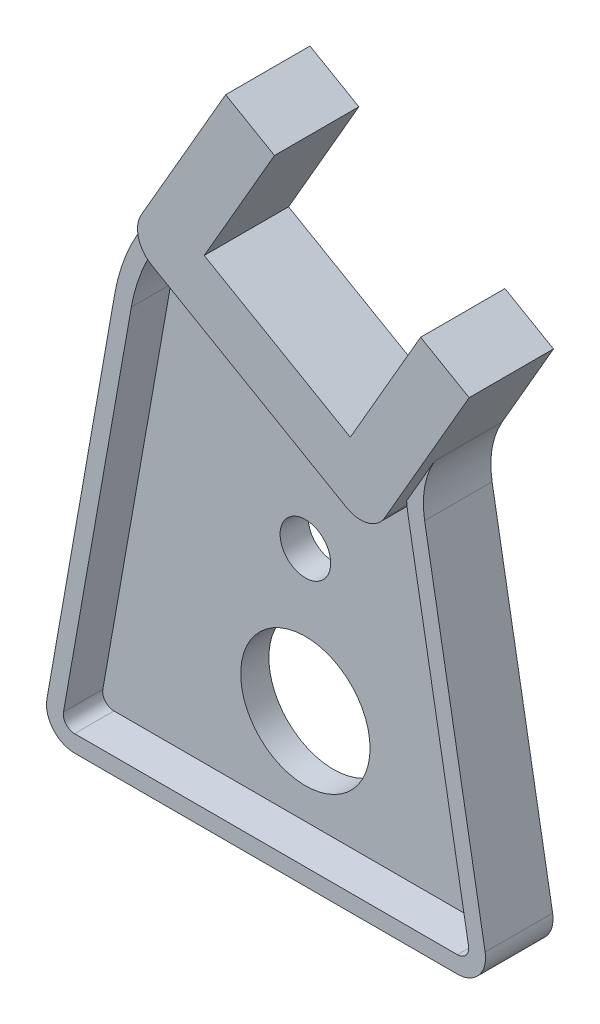
ISO-10303-21;
HEADER;
FILE_DESCRIPTION(('STEP AP214'),'2;1');
FILE_NAME('part.step','',(''),(''),'','','');
FILE_SCHEMA(('AUTOMOTIVE_DESIGN { 1 0 10303 214 1 1 1 1 }'));
ENDSEC;
DATA;
#1=APPLICATION_CONTEXT('core data for automotive mechanical design processes');
#2=APPLICATION_PROTOCOL_DEFINITION('international standard','automotive_design',2000,#1);
#3=PRODUCT_CONTEXT('',#1,'mechanical');
#4=PRODUCT('Part','Part','',(#3));
#5=PRODUCT_RELATED_PRODUCT_CATEGORY('part','',(#4));
#6=PRODUCT_DEFINITION_FORMATION('','',#4);
#7=PRODUCT_DEFINITION_CONTEXT('part definition',#1,'design');
#8=PRODUCT_DEFINITION('design','',#6,#7);
#9=PRODUCT_DEFINITION_SHAPE('','',#8);
#10=(LENGTH_UNIT() NAMED_UNIT(*) SI_UNIT(.MILLI.,.METRE.));
#11=(NAMED_UNIT(*) PLANE_ANGLE_UNIT() SI_UNIT($,.RADIAN.));
#12=(NAMED_UNIT(*) SI_UNIT($,.STERADIAN.) SOLID_ANGLE_UNIT());
#13=UNCERTAINTY_MEASURE_WITH_UNIT(LENGTH_MEASURE(1.E-05),#10,'distance_accuracy_value','');
#14=(GEOMETRIC_REPRESENTATION_CONTEXT(3) GLOBAL_UNCERTAINTY_ASSIGNED_CONTEXT((#13)) GLOBAL_UNIT_ASSIGNED_CONTEXT((#10,
#11,#12)) REPRESENTATION_CONTEXT('',''));
#15=CARTESIAN_POINT('',(0.,0.,0.));
#16=DIRECTION('',(0.,0.,1.));
#17=DIRECTION('',(1.,0.,0.));
#18=AXIS2_PLACEMENT_3D('',#15,#16,#17);
#19=CARTESIAN_POINT('',(0.,45.,12.));
#20=DIRECTION('',(0.,0.,-1.));
#21=DIRECTION('',(-1.,0.,0.));
#22=AXIS2_PLACEMENT_3D('',#19,#20,#21);
#23=CYLINDRICAL_SURFACE('',#22,4.5);
#24=CARTESIAN_POINT('',(0.,45.,0.));
#25=DIRECTION('',(0.,0.,1.));
#26=DIRECTION('',(1.,0.,0.));
#27=AXIS2_PLACEMENT_3D('',#24,#25,#26);
#28=CIRCLE('',#27,4.5);
#29=CARTESIAN_POINT('',(4.5,45.,0.));
#30=VERTEX_POINT('',#29);
#31=EDGE_CURVE('E350',#30,#30,#28,.T.);
#32=ORIENTED_EDGE('',*,*,#31,.F.);
#33=EDGE_LOOP('',(#32));
#34=FACE_BOUND('',#33,.T.);
#35=CARTESIAN_POINT('',(0.,45.,5.));
#36=DIRECTION('',(0.,0.,1.));
#37=DIRECTION('',(1.,0.,0.));
#38=AXIS2_PLACEMENT_3D('',#35,#36,#37);
#39=CIRCLE('',#38,4.5);
#40=CARTESIAN_POINT('',(4.5,45.,5.));
#41=VERTEX_POINT('',#40);
#42=EDGE_CURVE('E312',#41,#41,#39,.T.);
#43=ORIENTED_EDGE('',*,*,#42,.T.);
#44=EDGE_LOOP('',(#43));
#45=FACE_BOUND('',#44,.T.);
#46=ADVANCED_FACE('F41',(#34,#45),#23,.F.);
#47=CARTESIAN_POINT('',(0.,20.,12.));
#48=DIRECTION('',(0.,0.,-1.));
#49=DIRECTION('',(-1.,0.,0.));
#50=AXIS2_PLACEMENT_3D('',#47,#48,#49);
#51=CYLINDRICAL_SURFACE('',#50,11.5);
#52=CARTESIAN_POINT('',(0.,20.,0.));
#53=DIRECTION('',(0.,0.,1.));
#54=DIRECTION('',(1.,0.,0.));
#55=AXIS2_PLACEMENT_3D('',#52,#53,#54);
#56=CIRCLE('',#55,11.5);
#57=CARTESIAN_POINT('',(11.5,20.,0.));
#58=VERTEX_POINT('',#57);
#59=EDGE_CURVE('E318',#58,#58,#56,.T.);
#60=ORIENTED_EDGE('',*,*,#59,.F.);
#61=EDGE_LOOP('',(#60));
#62=FACE_BOUND('',#61,.T.);
#63=CARTESIAN_POINT('',(0.,20.,5.));
#64=DIRECTION('',(0.,0.,1.));
#65=DIRECTION('',(1.,0.,0.));
#66=AXIS2_PLACEMENT_3D('',#63,#64,#65);
#67=CIRCLE('',#66,11.5);
#68=CARTESIAN_POINT('',(11.5,20.,5.));
#69=VERTEX_POINT('',#68);
#70=EDGE_CURVE('E44',#69,#69,#67,.T.);
#71=ORIENTED_EDGE('',*,*,#70,.T.);
#72=EDGE_LOOP('',(#71));
#73=FACE_BOUND('',#72,.T.);
#74=ADVANCED_FACE('F555',(#62,#73),#51,.F.);
#75=CARTESIAN_POINT('',(-54.1549312273806,31.2663641220735,15.));
#76=DIRECTION('',(-0.866025403784441,0.499999999999996,0.));
#77=DIRECTION('',(-0.499999999999997,-0.866025403784441,0.));
#78=AXIS2_PLACEMENT_3D('',#75,#76,#77);
#79=PLANE('',#78);
#80=DIRECTION('',(0.499999999999996,0.866025403784441,0.));
#81=VECTOR('',#80,1.);
#82=CARTESIAN_POINT('',(-54.1549312273806,31.2663641220735,0.));
#83=LINE('',#82,#81);
#84=CARTESIAN_POINT('',(-22.7411868660834,85.6765654118211,0.));
#85=VERTEX_POINT('',#84);
#86=CARTESIAN_POINT('',(-4.17897858546452,117.827253254529,0.));
#87=VERTEX_POINT('',#86);
#88=EDGE_CURVE('E390',#85,#87,#83,.T.);
#89=ORIENTED_EDGE('',*,*,#88,.F.);
#90=DIRECTION('',(0.,0.,-1.));
#91=VECTOR('',#90,1.);
#92=CARTESIAN_POINT('',(-22.7411868660834,85.6765654118211,12.));
#93=LINE('',#92,#91);
#94=CARTESIAN_POINT('',(-22.7411868660834,85.6765654118211,12.));
#95=VERTEX_POINT('',#94);
#96=EDGE_CURVE('E374',#95,#85,#93,.T.);
#97=ORIENTED_EDGE('',*,*,#96,.F.);
#98=DIRECTION('',(0.499999999999996,0.866025403784441,0.));
#99=VECTOR('',#98,1.);
#100=CARTESIAN_POINT('',(-54.1549312273806,31.2663641220735,12.));
#101=LINE('',#100,#99);
#102=CARTESIAN_POINT('',(-19.1789785854643,91.846491140996,12.));
#103=VERTEX_POINT('',#102);
#104=EDGE_CURVE('E331',#95,#103,#101,.T.);
#105=ORIENTED_EDGE('',*,*,#104,.T.);
#106=DIRECTION('',(0.,0.,-1.));
#107=VECTOR('',#106,1.);
#108=CARTESIAN_POINT('',(-19.1789785854643,91.846491140996,15.));
#109=LINE('',#108,#107);
#110=CARTESIAN_POINT('',(-19.1789785854643,91.846491140996,15.));
#111=VERTEX_POINT('',#110);
#112=EDGE_CURVE('E11',#111,#103,#109,.T.);
#113=ORIENTED_EDGE('',*,*,#112,.F.);
#114=DIRECTION('',(0.499999999999996,0.866025403784441,0.));
#115=VECTOR('',#114,1.);
#116=CARTESIAN_POINT('',(-54.1549312273806,31.2663641220735,15.));
#117=LINE('',#116,#115);
#118=CARTESIAN_POINT('',(-4.17897858546452,117.827253254529,15.));
#119=VERTEX_POINT('',#118);
#120=EDGE_CURVE('E389',#111,#119,#117,.T.);
#121=ORIENTED_EDGE('',*,*,#120,.T.);
#122=DIRECTION('',(0.,0.,-1.));
#123=VECTOR('',#122,1.);
#124=CARTESIAN_POINT('',(-4.17897858546452,117.827253254529,15.));
#125=LINE('',#124,#123);
#126=EDGE_CURVE('E414',#119,#87,#125,.T.);
#127=ORIENTED_EDGE('',*,*,#126,.T.);
#128=EDGE_LOOP('',(#89,#97,#105,#113,#121,#127));
#129=FACE_BOUND('',#128,.T.);
#130=ADVANCED_FACE('F43',(#129),#79,.T.);
#131=CARTESIAN_POINT('',(-14.8488515665423,89.3464911409962,15.));
#132=DIRECTION('',(0.,0.,-1.));
#133=DIRECTION('',(-1.,0.,0.));
#134=AXIS2_PLACEMENT_3D('',#131,#132,#133);
#135=CYLINDRICAL_SURFACE('',#134,4.9999999999999);
#136=ORIENTED_EDGE('',*,*,#112,.T.);
#137=CARTESIAN_POINT('',(-14.8488515665423,89.3464911409962,12.));
#138=DIRECTION('',(0.,0.,1.));
#139=DIRECTION('',(1.,0.,0.));
#140=AXIS2_PLACEMENT_3D('',#137,#138,#139);
#141=CIRCLE('',#140,4.9999999999999);
#142=CARTESIAN_POINT('',(-18.8721898947694,86.3778637314644,12.));
#143=VERTEX_POINT('',#142);
#144=EDGE_CURVE('E335',#103,#143,#141,.T.);
#145=ORIENTED_EDGE('',*,*,#144,.T.);
#146=DIRECTION('',(0.,0.,1.));
#147=VECTOR('',#146,1.);
#148=CARTESIAN_POINT('',(-18.8721898947694,86.3778637314644,5.));
#149=LINE('',#148,#147);
#150=CARTESIAN_POINT('',(-18.8721898947694,86.3778637314644,5.));
#151=VERTEX_POINT('',#150);
#152=EDGE_CURVE('E280',#151,#143,#149,.T.);
#153=ORIENTED_EDGE('',*,*,#152,.F.);
#154=CARTESIAN_POINT('',(-14.8488515665423,89.3464911409962,5.));
#155=DIRECTION('',(0.,0.,-1.));
#156=DIRECTION('',(1.,0.,0.));
#157=AXIS2_PLACEMENT_3D('',#154,#155,#156);
#158=CIRCLE('',#157,5.00000000000019);
#159=CARTESIAN_POINT('',(-17.3488515665418,85.0163641220735,5.));
#160=VERTEX_POINT('',#159);
#161=EDGE_CURVE('E238',#160,#151,#158,.T.);
#162=ORIENTED_EDGE('',*,*,#161,.F.);
#163=DIRECTION('',(0.,0.,-1.));
#164=VECTOR('',#163,1.);
#165=CARTESIAN_POINT('',(-17.348851566542,85.0163641220738,15.));
#166=LINE('',#165,#164);
#167=CARTESIAN_POINT('',(-17.348851566542,85.0163641220738,15.));
#168=VERTEX_POINT('',#167);
#169=EDGE_CURVE('E49',#168,#160,#166,.T.);
#170=ORIENTED_EDGE('',*,*,#169,.F.);
#171=CARTESIAN_POINT('',(-14.8488515665423,89.3464911409962,15.));
#172=DIRECTION('',(0.,0.,1.));
#173=DIRECTION('',(1.,0.,0.));
#174=AXIS2_PLACEMENT_3D('',#171,#172,#173);
#175=CIRCLE('',#174,4.9999999999999);
#176=EDGE_CURVE('E393',#111,#168,#175,.T.);
#177=ORIENTED_EDGE('',*,*,#176,.F.);
#178=EDGE_LOOP('',(#136,#145,#153,#162,#170,#177));
#179=FACE_BOUND('',#178,.T.);
#180=ADVANCED_FACE('F475',(#179),#135,.T.);
#181=CARTESIAN_POINT('',(32.4759526419163,56.2500000000003,15.));
#182=DIRECTION('',(-0.499999999999996,-0.866025403784441,0.));
#183=DIRECTION('',(0.866025403784441,-0.499999999999996,0.));
#184=AXIS2_PLACEMENT_3D('',#181,#182,#183);
#185=PLANE('',#184);
#186=ORIENTED_EDGE('',*,*,#169,.T.);
#187=DIRECTION('',(-0.866025403784441,0.499999999999997,0.));
#188=VECTOR('',#187,1.);
#189=CARTESIAN_POINT('',(-17.3488515665417,85.0163641220737,5.));
#190=LINE('',#189,#188);
#191=CARTESIAN_POINT('',(17.2921645848359,65.0163641220738,5.));
#192=VERTEX_POINT('',#191);
#193=EDGE_CURVE('E233',#192,#160,#190,.T.);
#194=ORIENTED_EDGE('',*,*,#193,.F.);
#195=DIRECTION('',(0.,0.,-1.));
#196=VECTOR('',#195,1.);
#197=CARTESIAN_POINT('',(17.2921645848368,65.0163641220732,15.));
#198=LINE('',#197,#196);
#199=CARTESIAN_POINT('',(17.2921645848368,65.0163641220732,15.));
#200=VERTEX_POINT('',#199);
#201=EDGE_CURVE('E219',#200,#192,#198,.T.);
#202=ORIENTED_EDGE('',*,*,#201,.F.);
#203=DIRECTION('',(-0.866025403784441,0.499999999999996,0.));
#204=VECTOR('',#203,1.);
#205=CARTESIAN_POINT('',(32.4759526419163,56.2500000000003,15.));
#206=LINE('',#205,#204);
#207=EDGE_CURVE('E392',#200,#168,#206,.T.);
#208=ORIENTED_EDGE('',*,*,#207,.T.);
#209=EDGE_LOOP('',(#186,#194,#202,#208));
#210=FACE_BOUND('',#209,.T.);
#211=ADVANCED_FACE('F234',(#210),#185,.T.);
#212=CARTESIAN_POINT('',(19.7921645848368,69.346491140996,15.));
#213=DIRECTION('',(0.,0.,-1.));
#214=DIRECTION('',(-1.,0.,0.));
#215=AXIS2_PLACEMENT_3D('',#212,#213,#214);
#216=CYLINDRICAL_SURFACE('',#215,5.00000000000038);
#217=ORIENTED_EDGE('',*,*,#201,.T.);
#218=CARTESIAN_POINT('',(19.7921645848368,69.346491140996,5.));
#219=DIRECTION('',(0.,0.,-1.));
#220=DIRECTION('',(1.,0.,0.));
#221=AXIS2_PLACEMENT_3D('',#218,#219,#220);
#222=CIRCLE('',#221,5.00000000000041);
#223=CARTESIAN_POINT('',(24.1222916037574,66.8464911409923,5.));
#224=VERTEX_POINT('',#223);
#225=EDGE_CURVE('E223',#224,#192,#222,.T.);
#226=ORIENTED_EDGE('',*,*,#225,.F.);
#227=DIRECTION('',(0.,0.,-1.));
#228=VECTOR('',#227,1.);
#229=CARTESIAN_POINT('',(24.1222916037591,66.8464911409955,15.));
#230=LINE('',#229,#228);
#231=CARTESIAN_POINT('',(24.1222916037591,66.8464911409955,15.));
#232=VERTEX_POINT('',#231);
#233=EDGE_CURVE('E231',#232,#224,#230,.T.);
#234=ORIENTED_EDGE('',*,*,#233,.F.);
#235=CARTESIAN_POINT('',(19.7921645848368,69.346491140996,15.));
#236=DIRECTION('',(0.,0.,1.));
#237=DIRECTION('',(1.,0.,0.));
#238=AXIS2_PLACEMENT_3D('',#235,#236,#237);
#239=CIRCLE('',#238,5.00000000000038);
#240=EDGE_CURVE('E230',#200,#232,#239,.T.);
#241=ORIENTED_EDGE('',*,*,#240,.F.);
#242=EDGE_LOOP('',(#217,#226,#234,#241));
#243=FACE_BOUND('',#242,.T.);
#244=ADVANCED_FACE('F225',(#243),#216,.T.);
#245=CARTESIAN_POINT('',(-10.8536610381571,6.26636412207289,15.));
#246=DIRECTION('',(0.866025403784441,-0.499999999999995,0.));
#247=DIRECTION('',(0.499999999999995,0.866025403784441,0.));
#248=AXIS2_PLACEMENT_3D('',#245,#246,#247);
#249=PLANE('',#248);
#250=DIRECTION('',(0.,0.,-1.));
#251=VECTOR('',#250,1.);
#252=CARTESIAN_POINT('',(29.9790052785057,76.9906167910401,12.));
#253=LINE('',#252,#251);
#254=CARTESIAN_POINT('',(29.9790052785057,76.9906167910401,12.));
#255=VERTEX_POINT('',#254);
#256=CARTESIAN_POINT('',(29.9790052785057,76.9906167910401,0.));
#257=VERTEX_POINT('',#256);
#258=EDGE_CURVE('E378',#255,#257,#253,.T.);
#259=ORIENTED_EDGE('',*,*,#258,.T.);
#260=DIRECTION('',(-0.499999999999995,-0.866025403784441,0.));
#261=VECTOR('',#260,1.);
#262=CARTESIAN_POINT('',(-10.8536610381571,6.26636412207289,0.));
#263=LINE('',#262,#261);
#264=CARTESIAN_POINT('',(39.1222916037588,92.8272532545284,0.));
#265=VERTEX_POINT('',#264);
#266=EDGE_CURVE('E416',#265,#257,#263,.T.);
#267=ORIENTED_EDGE('',*,*,#266,.F.);
#268=DIRECTION('',(0.,0.,-1.));
#269=VECTOR('',#268,1.);
#270=CARTESIAN_POINT('',(39.1222916037588,92.8272532545284,15.));
#271=LINE('',#270,#269);
#272=CARTESIAN_POINT('',(39.1222916037588,92.8272532545284,15.));
#273=VERTEX_POINT('',#272);
#274=EDGE_CURVE('E441',#273,#265,#271,.T.);
#275=ORIENTED_EDGE('',*,*,#274,.F.);
#276=DIRECTION('',(-0.499999999999995,-0.866025403784441,0.));
#277=VECTOR('',#276,1.);
#278=CARTESIAN_POINT('',(-10.8536610381571,6.26636412207289,15.));
#279=LINE('',#278,#277);
#280=EDGE_CURVE('E400',#273,#232,#279,.T.);
#281=ORIENTED_EDGE('',*,*,#280,.T.);
#282=ORIENTED_EDGE('',*,*,#233,.T.);
#283=DIRECTION('',(-0.500000000000683,-0.866025403784044,0.));
#284=VECTOR('',#283,1.);
#285=CARTESIAN_POINT('',(25.0097459424172,68.3836071449457,5.));
#286=LINE('',#285,#284);
#287=CARTESIAN_POINT('',(25.0097459424172,68.3836071449457,5.));
#288=VERTEX_POINT('',#287);
#289=EDGE_CURVE('E244',#288,#224,#286,.T.);
#290=ORIENTED_EDGE('',*,*,#289,.F.);
#291=DIRECTION('',(0.,0.,1.));
#292=VECTOR('',#291,1.);
#293=CARTESIAN_POINT('',(25.0097459424172,68.3836071449457,5.));
#294=LINE('',#293,#292);
#295=CARTESIAN_POINT('',(25.0097459424172,68.3836071449457,12.));
#296=VERTEX_POINT('',#295);
#297=EDGE_CURVE('E296',#288,#296,#294,.T.);
#298=ORIENTED_EDGE('',*,*,#297,.T.);
#299=DIRECTION('',(-0.499999999999995,-0.866025403784441,0.));
#300=VECTOR('',#299,1.);
#301=CARTESIAN_POINT('',(-10.8536610381571,6.26636412207289,12.));
#302=LINE('',#301,#300);
#303=EDGE_CURVE('E61',#255,#296,#302,.T.);
#304=ORIENTED_EDGE('',*,*,#303,.F.);
#305=EDGE_LOOP('',(#259,#267,#275,#281,#282,#290,#298,#304));
#306=FACE_BOUND('',#305,.T.);
#307=ADVANCED_FACE('F450',(#306),#249,.T.);
#308=CARTESIAN_POINT('',(49.9759526419159,86.5608891324555,15.));
#309=DIRECTION('',(0.499999999999995,0.866025403784441,0.));
#310=DIRECTION('',(-0.866025403784441,0.499999999999995,0.));
#311=AXIS2_PLACEMENT_3D('',#308,#309,#310);
#312=PLANE('',#311);
#313=DIRECTION('',(0.866025403784441,-0.499999999999995,0.));
#314=VECTOR('',#313,1.);
#315=CARTESIAN_POINT('',(49.9759526419159,86.5608891324555,0.));
#316=LINE('',#315,#314);
#317=CARTESIAN_POINT('',(30.4903810567656,97.8108891324557,0.));
#318=VERTEX_POINT('',#317);
#319=EDGE_CURVE('E423',#318,#265,#316,.T.);
#320=ORIENTED_EDGE('',*,*,#319,.F.);
#321=DIRECTION('',(0.,0.,-1.));
#322=VECTOR('',#321,1.);
#323=CARTESIAN_POINT('',(30.4903810567656,97.8108891324557,15.));
#324=LINE('',#323,#322);
#325=CARTESIAN_POINT('',(30.4903810567656,97.8108891324557,15.));
#326=VERTEX_POINT('',#325);
#327=EDGE_CURVE('E445',#326,#318,#324,.T.);
#328=ORIENTED_EDGE('',*,*,#327,.F.);
#329=DIRECTION('',(0.866025403784441,-0.499999999999995,0.));
#330=VECTOR('',#329,1.);
#331=CARTESIAN_POINT('',(49.9759526419159,86.5608891324555,15.));
#332=LINE('',#331,#330);
#333=EDGE_CURVE('E399',#326,#273,#332,.T.);
#334=ORIENTED_EDGE('',*,*,#333,.T.);
#335=ORIENTED_EDGE('',*,*,#274,.T.);
#336=EDGE_LOOP('',(#320,#328,#334,#335));
#337=FACE_BOUND('',#336,.T.);
#338=ADVANCED_FACE('F460',(#337),#312,.T.);
#339=CARTESIAN_POINT('',(-19.4855715851504,11.2500000000002,15.));
#340=DIRECTION('',(-0.866025403784441,0.499999999999996,0.));
#341=DIRECTION('',(-0.499999999999996,-0.866025403784441,0.));
#342=AXIS2_PLACEMENT_3D('',#339,#340,#341);
#343=PLANE('',#342);
#344=DIRECTION('',(0.499999999999996,0.866025403784441,0.));
#345=VECTOR('',#344,1.);
#346=CARTESIAN_POINT('',(-19.4855715851504,11.2500000000002,0.));
#347=LINE('',#346,#345);
#348=CARTESIAN_POINT('',(17.9903810567657,76.1602540378446,0.));
#349=VERTEX_POINT('',#348);
#350=EDGE_CURVE('E424',#349,#318,#347,.T.);
#351=ORIENTED_EDGE('',*,*,#350,.F.);
#352=DIRECTION('',(0.,0.,-1.));
#353=VECTOR('',#352,1.);
#354=CARTESIAN_POINT('',(17.9903810567657,76.1602540378446,15.));
#355=LINE('',#354,#353);
#356=CARTESIAN_POINT('',(17.9903810567657,76.1602540378446,15.));
#357=VERTEX_POINT('',#356);
#358=EDGE_CURVE('E439',#357,#349,#355,.T.);
#359=ORIENTED_EDGE('',*,*,#358,.F.);
#360=DIRECTION('',(0.499999999999996,0.866025403784441,0.));
#361=VECTOR('',#360,1.);
#362=CARTESIAN_POINT('',(-19.4855715851504,11.2500000000002,15.));
#363=LINE('',#362,#361);
#364=EDGE_CURVE('E401',#357,#326,#363,.T.);
#365=ORIENTED_EDGE('',*,*,#364,.T.);
#366=ORIENTED_EDGE('',*,*,#327,.T.);
#367=EDGE_LOOP('',(#351,#359,#365,#366));
#368=FACE_BOUND('',#367,.T.);
#369=ADVANCED_FACE('F458',(#368),#343,.T.);
#370=CARTESIAN_POINT('',(37.4759526419161,64.9102540378444,15.));
#371=DIRECTION('',(0.499999999999997,0.866025403784441,0.));
#372=DIRECTION('',(-0.866025403784441,0.499999999999997,0.));
#373=AXIS2_PLACEMENT_3D('',#370,#371,#372);
#374=PLANE('',#373);
#375=DIRECTION('',(0.866025403784441,-0.499999999999997,0.));
#376=VECTOR('',#375,1.);
#377=CARTESIAN_POINT('',(37.4759526419161,64.9102540378444,0.));
#378=LINE('',#377,#376);
#379=CARTESIAN_POINT('',(-7.99038105676753,91.1602540378445,0.));
#380=VERTEX_POINT('',#379);
#381=EDGE_CURVE('E430',#380,#349,#378,.T.);
#382=ORIENTED_EDGE('',*,*,#381,.F.);
#383=DIRECTION('',(0.,0.,-1.));
#384=VECTOR('',#383,1.);
#385=CARTESIAN_POINT('',(-7.99038105676753,91.1602540378445,15.));
#386=LINE('',#385,#384);
#387=CARTESIAN_POINT('',(-7.99038105676753,91.1602540378445,15.));
#388=VERTEX_POINT('',#387);
#389=EDGE_CURVE('E437',#388,#380,#386,.T.);
#390=ORIENTED_EDGE('',*,*,#389,.F.);
#391=DIRECTION('',(0.866025403784441,-0.499999999999997,0.));
#392=VECTOR('',#391,1.);
#393=CARTESIAN_POINT('',(37.4759526419161,64.9102540378444,15.));
#394=LINE('',#393,#392);
#395=EDGE_CURVE('E408',#388,#357,#394,.T.);
#396=ORIENTED_EDGE('',*,*,#395,.T.);
#397=ORIENTED_EDGE('',*,*,#358,.T.);
#398=EDGE_LOOP('',(#382,#390,#396,#397));
#399=FACE_BOUND('',#398,.T.);
#400=ADVANCED_FACE('F464',(#399),#374,.T.);
#401=CARTESIAN_POINT('',(-45.4663336986836,26.25,15.));
#402=DIRECTION('',(0.866025403784441,-0.499999999999996,0.));
#403=DIRECTION('',(0.499999999999996,0.866025403784441,0.));
#404=AXIS2_PLACEMENT_3D('',#401,#402,#403);
#405=PLANE('',#404);
#406=DIRECTION('',(-0.499999999999996,-0.866025403784441,0.));
#407=VECTOR('',#406,1.);
#408=CARTESIAN_POINT('',(-45.4663336986836,26.25,0.));
#409=LINE('',#408,#407);
#410=CARTESIAN_POINT('',(4.50961894323237,112.810889132456,0.));
#411=VERTEX_POINT('',#410);
#412=EDGE_CURVE('E429',#411,#380,#409,.T.);
#413=ORIENTED_EDGE('',*,*,#412,.F.);
#414=DIRECTION('',(0.,0.,-1.));
#415=VECTOR('',#414,1.);
#416=CARTESIAN_POINT('',(4.50961894323237,112.810889132456,15.));
#417=LINE('',#416,#415);
#418=CARTESIAN_POINT('',(4.50961894323237,112.810889132456,15.));
#419=VERTEX_POINT('',#418);
#420=EDGE_CURVE('E436',#419,#411,#417,.T.);
#421=ORIENTED_EDGE('',*,*,#420,.F.);
#422=DIRECTION('',(-0.499999999999996,-0.866025403784441,0.));
#423=VECTOR('',#422,1.);
#424=CARTESIAN_POINT('',(-45.4663336986836,26.25,15.));
#425=LINE('',#424,#423);
#426=EDGE_CURVE('E407',#419,#388,#425,.T.);
#427=ORIENTED_EDGE('',*,*,#426,.T.);
#428=ORIENTED_EDGE('',*,*,#389,.T.);
#429=EDGE_LOOP('',(#413,#421,#427,#428));
#430=FACE_BOUND('',#429,.T.);
#431=ADVANCED_FACE('F467',(#430),#405,.T.);
#432=CARTESIAN_POINT('',(49.975952641916,86.5608891324555,15.));
#433=DIRECTION('',(0.499999999999996,0.866025403784441,0.));
#434=DIRECTION('',(-0.866025403784441,0.499999999999996,0.));
#435=AXIS2_PLACEMENT_3D('',#432,#433,#434);
#436=PLANE('',#435);
#437=DIRECTION('',(0.866025403784441,-0.499999999999996,0.));
#438=VECTOR('',#437,1.);
#439=CARTESIAN_POINT('',(49.975952641916,86.5608891324555,0.));
#440=LINE('',#439,#438);
#441=EDGE_CURVE('E395',#87,#411,#440,.T.);
#442=ORIENTED_EDGE('',*,*,#441,.F.);
#443=ORIENTED_EDGE('',*,*,#126,.F.);
#444=DIRECTION('',(0.866025403784441,-0.499999999999996,0.));
#445=VECTOR('',#444,1.);
#446=CARTESIAN_POINT('',(49.975952641916,86.5608891324555,15.));
#447=LINE('',#446,#445);
#448=EDGE_CURVE('E415',#119,#419,#447,.T.);
#449=ORIENTED_EDGE('',*,*,#448,.T.);
#450=ORIENTED_EDGE('',*,*,#420,.T.);
#451=EDGE_LOOP('',(#442,#443,#449,#450));
#452=FACE_BOUND('',#451,.T.);
#453=ADVANCED_FACE('F472',(#452),#436,.T.);
#454=CARTESIAN_POINT('',(0.,0.,15.));
#455=DIRECTION('',(0.,0.,1.));
#456=DIRECTION('',(1.,0.,0.));
#457=AXIS2_PLACEMENT_3D('',#454,#455,#456);
#458=PLANE('',#457);
#459=ORIENTED_EDGE('',*,*,#120,.F.);
#460=ORIENTED_EDGE('',*,*,#176,.T.);
#461=ORIENTED_EDGE('',*,*,#207,.F.);
#462=ORIENTED_EDGE('',*,*,#240,.T.);
#463=ORIENTED_EDGE('',*,*,#280,.F.);
#464=ORIENTED_EDGE('',*,*,#333,.F.);
#465=ORIENTED_EDGE('',*,*,#364,.F.);
#466=ORIENTED_EDGE('',*,*,#395,.F.);
#467=ORIENTED_EDGE('',*,*,#426,.F.);
#468=ORIENTED_EDGE('',*,*,#448,.F.);
#469=EDGE_LOOP('',(#459,#460,#461,#462,#463,#464,#465,#466,#467,#468));
#470=FACE_BOUND('',#469,.T.);
#471=ADVANCED_FACE('F452',(#470),#458,.T.);
#472=CARTESIAN_POINT('',(0.,0.,0.));
#473=DIRECTION('',(0.,0.,1.));
#474=DIRECTION('',(1.,0.,0.));
#475=AXIS2_PLACEMENT_3D('',#472,#473,#474);
#476=PLANE('',#475);
#477=ORIENTED_EDGE('',*,*,#266,.T.);
#478=CARTESIAN_POINT('',(42.9367881860438,69.5094373412723,0.));
#479=DIRECTION('',(0.,0.,1.));
#480=DIRECTION('',(1.,0.,0.));
#481=AXIS2_PLACEMENT_3D('',#478,#479,#480);
#482=CIRCLE('',#481,14.9623588995358);
#483=CARTESIAN_POINT('',(28.2017411384297,66.9112509847694,0.));
#484=VERTEX_POINT('',#483);
#485=EDGE_CURVE('E358',#257,#484,#482,.T.);
#486=ORIENTED_EDGE('',*,*,#485,.T.);
#487=DIRECTION('',(-0.173648177666913,0.984807753012211,0.));
#488=VECTOR('',#487,1.);
#489=CARTESIAN_POINT('',(38.7938524157176,6.84040286651256,0.));
#490=LINE('',#489,#488);
#491=CARTESIAN_POINT('',(38.9652708020894,5.86824088833388,0.));
#492=VERTEX_POINT('',#491);
#493=EDGE_CURVE('E356',#492,#484,#490,.T.);
#494=ORIENTED_EDGE('',*,*,#493,.F.);
#495=CARTESIAN_POINT('',(34.0412320370289,4.99999999999999,0.));
#496=DIRECTION('',(0.,0.,1.));
#497=DIRECTION('',(1.,0.,0.));
#498=AXIS2_PLACEMENT_3D('',#495,#496,#497);
#499=CIRCLE('',#498,4.99999999999964);
#500=CARTESIAN_POINT('',(34.0412320370289,0.,0.));
#501=VERTEX_POINT('',#500);
#502=EDGE_CURVE('E351',#501,#492,#499,.T.);
#503=ORIENTED_EDGE('',*,*,#502,.F.);
#504=DIRECTION('',(-1.,0.,0.));
#505=VECTOR('',#504,1.);
#506=CARTESIAN_POINT('',(0.,0.,0.));
#507=LINE('',#506,#505);
#508=CARTESIAN_POINT('',(-34.0412320370289,0.,0.));
#509=VERTEX_POINT('',#508);
#510=EDGE_CURVE('E348',#501,#509,#507,.T.);
#511=ORIENTED_EDGE('',*,*,#510,.T.);
#512=CARTESIAN_POINT('',(-34.0412320370289,5.,0.));
#513=DIRECTION('',(0.,0.,1.));
#514=DIRECTION('',(1.,0.,0.));
#515=AXIS2_PLACEMENT_3D('',#512,#513,#514);
#516=CIRCLE('',#515,4.99999999999939);
#517=CARTESIAN_POINT('',(-38.9652708020888,5.86824088833411,0.));
#518=VERTEX_POINT('',#517);
#519=EDGE_CURVE('E323',#518,#509,#516,.T.);
#520=ORIENTED_EDGE('',*,*,#519,.F.);
#521=DIRECTION('',(0.173648177666923,0.984807753012209,0.));
#522=VECTOR('',#521,1.);
#523=CARTESIAN_POINT('',(-38.793852415717,6.84040286651287,0.));
#524=LINE('',#523,#522);
#525=CARTESIAN_POINT('',(-26.9061956072052,74.2586548024835,0.));
#526=VERTEX_POINT('',#525);
#527=EDGE_CURVE('E364',#518,#526,#524,.T.);
#528=ORIENTED_EDGE('',*,*,#527,.T.);
#529=CARTESIAN_POINT('',(7.55759505036464,68.1556118310508,0.));
#530=DIRECTION('',(0.,0.,1.));
#531=DIRECTION('',(1.,0.,0.));
#532=AXIS2_PLACEMENT_3D('',#529,#530,#531);
#533=CIRCLE('',#532,34.9999999999995);
#534=EDGE_CURVE('E362',#85,#526,#533,.T.);
#535=ORIENTED_EDGE('',*,*,#534,.F.);
#536=ORIENTED_EDGE('',*,*,#88,.T.);
#537=ORIENTED_EDGE('',*,*,#441,.T.);
#538=ORIENTED_EDGE('',*,*,#412,.T.);
#539=ORIENTED_EDGE('',*,*,#381,.T.);
#540=ORIENTED_EDGE('',*,*,#350,.T.);
#541=ORIENTED_EDGE('',*,*,#319,.T.);
#542=EDGE_LOOP('',(#477,#486,#494,#503,#511,#520,#528,#535,#536,#537,#538,#539,#540,#541));
#543=FACE_BOUND('',#542,.T.);
#544=ORIENTED_EDGE('',*,*,#59,.T.);
#545=EDGE_LOOP('',(#544));
#546=FACE_BOUND('',#545,.T.);
#547=ORIENTED_EDGE('',*,*,#31,.T.);
#548=EDGE_LOOP('',(#547));
#549=FACE_BOUND('',#548,.T.);
#550=ADVANCED_FACE('F513',(#543,#546,#549),#476,.F.);
#551=CARTESIAN_POINT('',(0.,0.,12.));
#552=DIRECTION('',(0.,-1.,0.));
#553=DIRECTION('',(0.,0.,-1.));
#554=AXIS2_PLACEMENT_3D('',#551,#552,#553);
#555=PLANE('',#554);
#556=ORIENTED_EDGE('',*,*,#510,.F.);
#557=DIRECTION('',(0.,0.,-1.));
#558=VECTOR('',#557,1.);
#559=CARTESIAN_POINT('',(34.0412320370289,0.,12.));
#560=LINE('',#559,#558);
#561=CARTESIAN_POINT('',(34.0412320370289,0.,12.));
#562=VERTEX_POINT('',#561);
#563=EDGE_CURVE('E384',#562,#501,#560,.T.);
#564=ORIENTED_EDGE('',*,*,#563,.F.);
#565=DIRECTION('',(-1.,0.,0.));
#566=VECTOR('',#565,1.);
#567=CARTESIAN_POINT('',(0.,0.,12.));
#568=LINE('',#567,#566);
#569=CARTESIAN_POINT('',(-34.0412320370289,0.,12.));
#570=VERTEX_POINT('',#569);
#571=EDGE_CURVE('E317',#562,#570,#568,.T.);
#572=ORIENTED_EDGE('',*,*,#571,.T.);
#573=DIRECTION('',(0.,0.,-1.));
#574=VECTOR('',#573,1.);
#575=CARTESIAN_POINT('',(-34.0412320370289,0.,12.));
#576=LINE('',#575,#574);
#577=EDGE_CURVE('E343',#570,#509,#576,.T.);
#578=ORIENTED_EDGE('',*,*,#577,.T.);
#579=EDGE_LOOP('',(#556,#564,#572,#578));
#580=FACE_BOUND('',#579,.T.);
#581=ADVANCED_FACE('F532',(#580),#555,.T.);
#582=CARTESIAN_POINT('',(34.0412320370289,4.99999999999999,12.));
#583=DIRECTION('',(0.,0.,-1.));
#584=DIRECTION('',(-1.,0.,0.));
#585=AXIS2_PLACEMENT_3D('',#582,#583,#584);
#586=CYLINDRICAL_SURFACE('',#585,4.99999999999964);
#587=ORIENTED_EDGE('',*,*,#502,.T.);
#588=DIRECTION('',(0.,0.,-1.));
#589=VECTOR('',#588,1.);
#590=CARTESIAN_POINT('',(38.9652708020894,5.86824088833388,12.));
#591=LINE('',#590,#589);
#592=CARTESIAN_POINT('',(38.9652708020894,5.86824088833388,12.));
#593=VERTEX_POINT('',#592);
#594=EDGE_CURVE('E385',#593,#492,#591,.T.);
#595=ORIENTED_EDGE('',*,*,#594,.F.);
#596=CARTESIAN_POINT('',(34.0412320370289,4.99999999999999,12.));
#597=DIRECTION('',(0.,0.,1.));
#598=DIRECTION('',(1.,0.,0.));
#599=AXIS2_PLACEMENT_3D('',#596,#597,#598);
#600=CIRCLE('',#599,4.99999999999964);
#601=EDGE_CURVE('E325',#562,#593,#600,.T.);
#602=ORIENTED_EDGE('',*,*,#601,.F.);
#603=ORIENTED_EDGE('',*,*,#563,.T.);
#604=EDGE_LOOP('',(#587,#595,#602,#603));
#605=FACE_BOUND('',#604,.T.);
#606=ADVANCED_FACE('F537',(#605),#586,.T.);
#607=CARTESIAN_POINT('',(38.7938524157176,6.84040286651256,12.));
#608=DIRECTION('',(-0.984807753012211,-0.173648177666913,0.));
#609=DIRECTION('',(0.173648177666913,-0.984807753012211,0.));
#610=AXIS2_PLACEMENT_3D('',#607,#608,#609);
#611=PLANE('',#610);
#612=ORIENTED_EDGE('',*,*,#493,.T.);
#613=DIRECTION('',(0.,0.,-1.));
#614=VECTOR('',#613,1.);
#615=CARTESIAN_POINT('',(28.2017411384297,66.9112509847694,12.));
#616=LINE('',#615,#614);
#617=CARTESIAN_POINT('',(28.2017411384297,66.9112509847694,12.));
#618=VERTEX_POINT('',#617);
#619=EDGE_CURVE('E379',#618,#484,#616,.T.);
#620=ORIENTED_EDGE('',*,*,#619,.F.);
#621=DIRECTION('',(-0.173648177666913,0.984807753012211,0.));
#622=VECTOR('',#621,1.);
#623=CARTESIAN_POINT('',(38.7938524157176,6.84040286651256,12.));
#624=LINE('',#623,#622);
#625=EDGE_CURVE('E326',#593,#618,#624,.T.);
#626=ORIENTED_EDGE('',*,*,#625,.F.);
#627=ORIENTED_EDGE('',*,*,#594,.T.);
#628=EDGE_LOOP('',(#612,#620,#626,#627));
#629=FACE_BOUND('',#628,.T.);
#630=ADVANCED_FACE('F545',(#629),#611,.F.);
#631=CARTESIAN_POINT('',(42.9367881860438,69.5094373412723,12.));
#632=DIRECTION('',(0.,0.,-1.));
#633=DIRECTION('',(-1.,0.,0.));
#634=AXIS2_PLACEMENT_3D('',#631,#632,#633);
#635=CYLINDRICAL_SURFACE('',#634,14.9623588995358);
#636=ORIENTED_EDGE('',*,*,#485,.F.);
#637=ORIENTED_EDGE('',*,*,#258,.F.);
#638=CARTESIAN_POINT('',(42.9367881860438,69.5094373412723,12.));
#639=DIRECTION('',(0.,0.,1.));
#640=DIRECTION('',(1.,0.,0.));
#641=AXIS2_PLACEMENT_3D('',#638,#639,#640);
#642=CIRCLE('',#641,14.9623588995358);
#643=EDGE_CURVE('E327',#255,#618,#642,.T.);
#644=ORIENTED_EDGE('',*,*,#643,.T.);
#645=ORIENTED_EDGE('',*,*,#619,.T.);
#646=EDGE_LOOP('',(#636,#637,#644,#645));
#647=FACE_BOUND('',#646,.T.);
#648=ADVANCED_FACE('F511',(#647),#635,.F.);
#649=CARTESIAN_POINT('',(7.55759505036464,68.1556118310508,12.));
#650=DIRECTION('',(0.,0.,-1.));
#651=DIRECTION('',(-1.,0.,0.));
#652=AXIS2_PLACEMENT_3D('',#649,#650,#651);
#653=CYLINDRICAL_SURFACE('',#652,34.9999999999995);
#654=ORIENTED_EDGE('',*,*,#534,.T.);
#655=DIRECTION('',(0.,0.,-1.));
#656=VECTOR('',#655,1.);
#657=CARTESIAN_POINT('',(-26.9061956072052,74.2586548024835,12.));
#658=LINE('',#657,#656);
#659=CARTESIAN_POINT('',(-26.9061956072052,74.2586548024835,12.));
#660=VERTEX_POINT('',#659);
#661=EDGE_CURVE('E373',#660,#526,#658,.T.);
#662=ORIENTED_EDGE('',*,*,#661,.F.);
#663=CARTESIAN_POINT('',(7.55759505036464,68.1556118310508,12.));
#664=DIRECTION('',(0.,0.,1.));
#665=DIRECTION('',(1.,0.,0.));
#666=AXIS2_PLACEMENT_3D('',#663,#664,#665);
#667=CIRCLE('',#666,34.9999999999995);
#668=EDGE_CURVE('E340',#95,#660,#667,.T.);
#669=ORIENTED_EDGE('',*,*,#668,.F.);
#670=ORIENTED_EDGE('',*,*,#96,.T.);
#671=EDGE_LOOP('',(#654,#662,#669,#670));
#672=FACE_BOUND('',#671,.T.);
#673=ADVANCED_FACE('F519',(#672),#653,.T.);
#674=CARTESIAN_POINT('',(-38.793852415717,6.84040286651287,12.));
#675=DIRECTION('',(-0.984807753012209,0.173648177666923,0.));
#676=DIRECTION('',(-0.173648177666923,-0.984807753012209,0.));
#677=AXIS2_PLACEMENT_3D('',#674,#675,#676);
#678=PLANE('',#677);
#679=ORIENTED_EDGE('',*,*,#527,.F.);
#680=DIRECTION('',(0.,0.,-1.));
#681=VECTOR('',#680,1.);
#682=CARTESIAN_POINT('',(-38.9652708020888,5.86824088833411,12.));
#683=LINE('',#682,#681);
#684=CARTESIAN_POINT('',(-38.9652708020888,5.86824088833411,12.));
#685=VERTEX_POINT('',#684);
#686=EDGE_CURVE('E371',#685,#518,#683,.T.);
#687=ORIENTED_EDGE('',*,*,#686,.F.);
#688=DIRECTION('',(0.173648177666923,0.984807753012209,0.));
#689=VECTOR('',#688,1.);
#690=CARTESIAN_POINT('',(-38.793852415717,6.84040286651287,12.));
#691=LINE('',#690,#689);
#692=EDGE_CURVE('E337',#685,#660,#691,.T.);
#693=ORIENTED_EDGE('',*,*,#692,.T.);
#694=ORIENTED_EDGE('',*,*,#661,.T.);
#695=EDGE_LOOP('',(#679,#687,#693,#694));
#696=FACE_BOUND('',#695,.T.);
#697=ADVANCED_FACE('F530',(#696),#678,.T.);
#698=CARTESIAN_POINT('',(-34.0412320370289,5.,12.));
#699=DIRECTION('',(0.,0.,-1.));
#700=DIRECTION('',(-1.,0.,0.));
#701=AXIS2_PLACEMENT_3D('',#698,#699,#700);
#702=CYLINDRICAL_SURFACE('',#701,4.99999999999939);
#703=ORIENTED_EDGE('',*,*,#519,.T.);
#704=ORIENTED_EDGE('',*,*,#577,.F.);
#705=CARTESIAN_POINT('',(-34.0412320370289,5.,12.));
#706=DIRECTION('',(0.,0.,1.));
#707=DIRECTION('',(1.,0.,0.));
#708=AXIS2_PLACEMENT_3D('',#705,#706,#707);
#709=CIRCLE('',#708,4.99999999999939);
#710=EDGE_CURVE('E345',#685,#570,#709,.T.);
#711=ORIENTED_EDGE('',*,*,#710,.F.);
#712=ORIENTED_EDGE('',*,*,#686,.T.);
#713=EDGE_LOOP('',(#703,#704,#711,#712));
#714=FACE_BOUND('',#713,.T.);
#715=ADVANCED_FACE('F535',(#714),#702,.T.);
#716=CARTESIAN_POINT('',(0.,0.,12.));
#717=DIRECTION('',(0.,0.,1.));
#718=DIRECTION('',(1.,0.,0.));
#719=AXIS2_PLACEMENT_3D('',#716,#717,#718);
#720=PLANE('',#719);
#721=CARTESIAN_POINT('',(42.9367881860438,69.5094373412723,12.));
#722=DIRECTION('',(0.,0.,-1.));
#723=DIRECTION('',(1.,0.,0.));
#724=AXIS2_PLACEMENT_3D('',#721,#722,#723);
#725=CIRCLE('',#724,17.9623588995358);
#726=CARTESIAN_POINT('',(25.2473178793931,66.3903064517687,12.));
#727=VERTEX_POINT('',#726);
#728=EDGE_CURVE('E246',#727,#296,#725,.T.);
#729=ORIENTED_EDGE('',*,*,#728,.F.);
#730=DIRECTION('',(-0.173648177666918,0.98480775301221,0.));
#731=VECTOR('',#730,1.);
#732=CARTESIAN_POINT('',(25.2473178793931,66.3903064517687,12.));
#733=LINE('',#732,#731);
#734=CARTESIAN_POINT('',(36.0108475430531,5.34729635533354,12.));
#735=VERTEX_POINT('',#734);
#736=EDGE_CURVE('E248',#735,#727,#733,.T.);
#737=ORIENTED_EDGE('',*,*,#736,.F.);
#738=CARTESIAN_POINT('',(34.0412320370289,4.99999999999999,12.));
#739=DIRECTION('',(0.,0.,1.));
#740=DIRECTION('',(1.,0.,0.));
#741=AXIS2_PLACEMENT_3D('',#738,#739,#740);
#742=CIRCLE('',#741,1.99999999999982);
#743=CARTESIAN_POINT('',(34.0412320370289,3.00000000000017,12.));
#744=VERTEX_POINT('',#743);
#745=EDGE_CURVE('E291',#744,#735,#742,.T.);
#746=ORIENTED_EDGE('',*,*,#745,.F.);
#747=DIRECTION('',(1.,0.,0.));
#748=VECTOR('',#747,1.);
#749=CARTESIAN_POINT('',(34.0412320370289,2.99999999999999,12.));
#750=LINE('',#749,#748);
#751=CARTESIAN_POINT('',(-34.0412320370289,3.00000000000061,12.));
#752=VERTEX_POINT('',#751);
#753=EDGE_CURVE('E289',#752,#744,#750,.T.);
#754=ORIENTED_EDGE('',*,*,#753,.F.);
#755=CARTESIAN_POINT('',(-34.0412320370289,5.,12.));
#756=DIRECTION('',(0.,0.,1.));
#757=DIRECTION('',(1.,0.,0.));
#758=AXIS2_PLACEMENT_3D('',#755,#756,#757);
#759=CIRCLE('',#758,1.99999999999907);
#760=CARTESIAN_POINT('',(-36.0108475430525,5.34729635533339,12.));
#761=VERTEX_POINT('',#760);
#762=EDGE_CURVE('E290',#761,#752,#759,.T.);
#763=ORIENTED_EDGE('',*,*,#762,.F.);
#764=DIRECTION('',(-0.173648166153153,-0.984807755042398,0.));
#765=VECTOR('',#764,1.);
#766=CARTESIAN_POINT('',(-36.0108475430522,5.34729635533334,12.));
#767=LINE('',#766,#765);
#768=CARTESIAN_POINT('',(-23.9521564079851,73.7355368335036,12.));
#769=VERTEX_POINT('',#768);
#770=EDGE_CURVE('E282',#769,#761,#767,.T.);
#771=ORIENTED_EDGE('',*,*,#770,.F.);
#772=CARTESIAN_POINT('',(7.55759505036464,68.1556118310508,12.));
#773=DIRECTION('',(0.,0.,1.));
#774=DIRECTION('',(1.,0.,0.));
#775=AXIS2_PLACEMENT_3D('',#772,#773,#774);
#776=CIRCLE('',#775,31.9999999999995);
#777=CARTESIAN_POINT('',(-20.1431099757721,84.1765650191396,12.));
#778=VERTEX_POINT('',#777);
#779=EDGE_CURVE('E283',#778,#769,#776,.T.);
#780=ORIENTED_EDGE('',*,*,#779,.F.);
#781=DIRECTION('',(-0.499999904658218,-0.866025458830035,0.));
#782=VECTOR('',#781,1.);
#783=CARTESIAN_POINT('',(-20.1431099757721,84.1765650191396,12.));
#784=LINE('',#783,#782);
#785=EDGE_CURVE('E279',#143,#778,#784,.T.);
#786=ORIENTED_EDGE('',*,*,#785,.F.);
#787=ORIENTED_EDGE('',*,*,#144,.F.);
#788=ORIENTED_EDGE('',*,*,#104,.F.);
#789=ORIENTED_EDGE('',*,*,#668,.T.);
#790=ORIENTED_EDGE('',*,*,#692,.F.);
#791=ORIENTED_EDGE('',*,*,#710,.T.);
#792=ORIENTED_EDGE('',*,*,#571,.F.);
#793=ORIENTED_EDGE('',*,*,#601,.T.);
#794=ORIENTED_EDGE('',*,*,#625,.T.);
#795=ORIENTED_EDGE('',*,*,#643,.F.);
#796=ORIENTED_EDGE('',*,*,#303,.T.);
#797=EDGE_LOOP('',(#729,#737,#746,#754,#763,#771,#780,#786,#787,#788,#789,#790,#791,#792,#793,
#794,#795,#796));
#798=FACE_BOUND('',#797,.T.);
#799=ADVANCED_FACE('F508',(#798),#720,.T.);
#800=CARTESIAN_POINT('',(42.9367881860438,69.5094373412723,5.));
#801=DIRECTION('',(0.,0.,1.));
#802=DIRECTION('',(1.,0.,0.));
#803=AXIS2_PLACEMENT_3D('',#800,#801,#802);
#804=CYLINDRICAL_SURFACE('',#803,17.9623588995358);
#805=ORIENTED_EDGE('',*,*,#728,.T.);
#806=ORIENTED_EDGE('',*,*,#297,.F.);
#807=CARTESIAN_POINT('',(42.9367881860438,69.5094373412723,5.));
#808=DIRECTION('',(0.,0.,-1.));
#809=DIRECTION('',(1.,0.,0.));
#810=AXIS2_PLACEMENT_3D('',#807,#808,#809);
#811=CIRCLE('',#810,17.9623588995358);
#812=CARTESIAN_POINT('',(25.2473178793931,66.3903064517687,5.));
#813=VERTEX_POINT('',#812);
#814=EDGE_CURVE('E273',#813,#288,#811,.T.);
#815=ORIENTED_EDGE('',*,*,#814,.F.);
#816=DIRECTION('',(0.,0.,1.));
#817=VECTOR('',#816,1.);
#818=CARTESIAN_POINT('',(25.2473178793931,66.3903064517687,5.));
#819=LINE('',#818,#817);
#820=EDGE_CURVE('E299',#813,#727,#819,.T.);
#821=ORIENTED_EDGE('',*,*,#820,.T.);
#822=EDGE_LOOP('',(#805,#806,#815,#821));
#823=FACE_BOUND('',#822,.T.);
#824=ADVANCED_FACE('F506',(#823),#804,.T.);
#825=CARTESIAN_POINT('',(25.2473178793931,66.3903064517687,5.));
#826=DIRECTION('',(0.98480775301221,0.173648177666918,0.));
#827=DIRECTION('',(-0.173648177666918,0.98480775301221,0.));
#828=AXIS2_PLACEMENT_3D('',#825,#826,#827);
#829=PLANE('',#828);
#830=ORIENTED_EDGE('',*,*,#736,.T.);
#831=ORIENTED_EDGE('',*,*,#820,.F.);
#832=DIRECTION('',(-0.173648177666918,0.98480775301221,0.));
#833=VECTOR('',#832,1.);
#834=CARTESIAN_POINT('',(25.2473178793931,66.3903064517687,5.));
#835=LINE('',#834,#833);
#836=CARTESIAN_POINT('',(36.0108475430531,5.34729635533354,5.));
#837=VERTEX_POINT('',#836);
#838=EDGE_CURVE('E271',#837,#813,#835,.T.);
#839=ORIENTED_EDGE('',*,*,#838,.F.);
#840=DIRECTION('',(0.,0.,1.));
#841=VECTOR('',#840,1.);
#842=CARTESIAN_POINT('',(36.0108475430531,5.34729635533354,5.));
#843=LINE('',#842,#841);
#844=EDGE_CURVE('E305',#837,#735,#843,.T.);
#845=ORIENTED_EDGE('',*,*,#844,.T.);
#846=EDGE_LOOP('',(#830,#831,#839,#845));
#847=FACE_BOUND('',#846,.T.);
#848=ADVANCED_FACE('F505',(#847),#829,.F.);
#849=CARTESIAN_POINT('',(34.0412320370289,4.99999999999999,5.));
#850=DIRECTION('',(0.,0.,1.));
#851=DIRECTION('',(1.,0.,0.));
#852=AXIS2_PLACEMENT_3D('',#849,#850,#851);
#853=CYLINDRICAL_SURFACE('',#852,1.99999999999982);
#854=ORIENTED_EDGE('',*,*,#745,.T.);
#855=ORIENTED_EDGE('',*,*,#844,.F.);
#856=CARTESIAN_POINT('',(34.0412320370289,4.99999999999999,5.));
#857=DIRECTION('',(0.,0.,1.));
#858=DIRECTION('',(1.,0.,0.));
#859=AXIS2_PLACEMENT_3D('',#856,#857,#858);
#860=CIRCLE('',#859,1.99999999999982);
#861=CARTESIAN_POINT('',(34.0412320370289,3.00000000000017,5.));
#862=VERTEX_POINT('',#861);
#863=EDGE_CURVE('E268',#862,#837,#860,.T.);
#864=ORIENTED_EDGE('',*,*,#863,.F.);
#865=DIRECTION('',(0.,0.,1.));
#866=VECTOR('',#865,1.);
#867=CARTESIAN_POINT('',(34.0412320370289,3.00000000000017,5.));
#868=LINE('',#867,#866);
#869=EDGE_CURVE('E303',#862,#744,#868,.T.);
#870=ORIENTED_EDGE('',*,*,#869,.T.);
#871=EDGE_LOOP('',(#854,#855,#864,#870));
#872=FACE_BOUND('',#871,.T.);
#873=ADVANCED_FACE('F499',(#872),#853,.F.);
#874=CARTESIAN_POINT('',(34.0412320370289,2.99999999999999,5.));
#875=DIRECTION('',(0.,-1.,0.));
#876=DIRECTION('',(1.,0.,0.));
#877=AXIS2_PLACEMENT_3D('',#874,#875,#876);
#878=PLANE('',#877);
#879=ORIENTED_EDGE('',*,*,#753,.T.);
#880=ORIENTED_EDGE('',*,*,#869,.F.);
#881=DIRECTION('',(1.,0.,0.));
#882=VECTOR('',#881,1.);
#883=CARTESIAN_POINT('',(34.0412320370289,2.99999999999999,5.));
#884=LINE('',#883,#882);
#885=CARTESIAN_POINT('',(-34.0412320370289,3.00000000000061,5.));
#886=VERTEX_POINT('',#885);
#887=EDGE_CURVE('E264',#886,#862,#884,.T.);
#888=ORIENTED_EDGE('',*,*,#887,.F.);
#889=DIRECTION('',(0.,0.,1.));
#890=VECTOR('',#889,1.);
#891=CARTESIAN_POINT('',(-34.0412320370289,3.00000000000061,5.));
#892=LINE('',#891,#890);
#893=EDGE_CURVE('E308',#886,#752,#892,.T.);
#894=ORIENTED_EDGE('',*,*,#893,.T.);
#895=EDGE_LOOP('',(#879,#880,#888,#894));
#896=FACE_BOUND('',#895,.T.);
#897=ADVANCED_FACE('F493',(#896),#878,.F.);
#898=CARTESIAN_POINT('',(-34.0412320370289,5.,5.));
#899=DIRECTION('',(0.,0.,1.));
#900=DIRECTION('',(1.,0.,0.));
#901=AXIS2_PLACEMENT_3D('',#898,#899,#900);
#902=CYLINDRICAL_SURFACE('',#901,1.99999999999907);
#903=ORIENTED_EDGE('',*,*,#762,.T.);
#904=ORIENTED_EDGE('',*,*,#893,.F.);
#905=CARTESIAN_POINT('',(-34.0412320370289,5.,5.));
#906=DIRECTION('',(0.,0.,1.));
#907=DIRECTION('',(1.,0.,0.));
#908=AXIS2_PLACEMENT_3D('',#905,#906,#907);
#909=CIRCLE('',#908,1.99999999999907);
#910=CARTESIAN_POINT('',(-36.0108475430525,5.34729635533339,5.));
#911=VERTEX_POINT('',#910);
#912=EDGE_CURVE('E265',#911,#886,#909,.T.);
#913=ORIENTED_EDGE('',*,*,#912,.F.);
#914=DIRECTION('',(0.,0.,1.));
#915=VECTOR('',#914,1.);
#916=CARTESIAN_POINT('',(-36.0108475430525,5.34729635533339,5.));
#917=LINE('',#916,#915);
#918=EDGE_CURVE('E306',#911,#761,#917,.T.);
#919=ORIENTED_EDGE('',*,*,#918,.T.);
#920=EDGE_LOOP('',(#903,#904,#913,#919));
#921=FACE_BOUND('',#920,.T.);
#922=ADVANCED_FACE('F489',(#921),#902,.F.);
#923=CARTESIAN_POINT('',(-36.0108475430522,5.34729635533334,5.));
#924=DIRECTION('',(-0.984807755042398,0.173648166153153,0.));
#925=DIRECTION('',(-0.173648166153153,-0.984807755042398,0.));
#926=AXIS2_PLACEMENT_3D('',#923,#924,#925);
#927=PLANE('',#926);
#928=ORIENTED_EDGE('',*,*,#770,.T.);
#929=ORIENTED_EDGE('',*,*,#918,.F.);
#930=DIRECTION('',(-0.173648166153153,-0.984807755042398,0.));
#931=VECTOR('',#930,1.);
#932=CARTESIAN_POINT('',(-36.0108475430522,5.34729635533334,5.));
#933=LINE('',#932,#931);
#934=CARTESIAN_POINT('',(-23.9521564079851,73.7355368335036,5.));
#935=VERTEX_POINT('',#934);
#936=EDGE_CURVE('E259',#935,#911,#933,.T.);
#937=ORIENTED_EDGE('',*,*,#936,.F.);
#938=DIRECTION('',(0.,0.,1.));
#939=VECTOR('',#938,1.);
#940=CARTESIAN_POINT('',(-23.9521564079851,73.7355368335036,5.));
#941=LINE('',#940,#939);
#942=EDGE_CURVE('E309',#935,#769,#941,.T.);
#943=ORIENTED_EDGE('',*,*,#942,.T.);
#944=EDGE_LOOP('',(#928,#929,#937,#943));
#945=FACE_BOUND('',#944,.T.);
#946=ADVANCED_FACE('F486',(#945),#927,.F.);
#947=CARTESIAN_POINT('',(7.55759505036464,68.1556118310508,5.));
#948=DIRECTION('',(0.,0.,1.));
#949=DIRECTION('',(1.,0.,0.));
#950=AXIS2_PLACEMENT_3D('',#947,#948,#949);
#951=CYLINDRICAL_SURFACE('',#950,31.9999999999995);
#952=ORIENTED_EDGE('',*,*,#779,.T.);
#953=ORIENTED_EDGE('',*,*,#942,.F.);
#954=CARTESIAN_POINT('',(7.55759505036464,68.1556118310508,5.));
#955=DIRECTION('',(0.,0.,1.));
#956=DIRECTION('',(1.,0.,0.));
#957=AXIS2_PLACEMENT_3D('',#954,#955,#956);
#958=CIRCLE('',#957,31.9999999999995);
#959=CARTESIAN_POINT('',(-20.1431099757721,84.1765650191396,5.));
#960=VERTEX_POINT('',#959);
#961=EDGE_CURVE('E258',#960,#935,#958,.T.);
#962=ORIENTED_EDGE('',*,*,#961,.F.);
#963=DIRECTION('',(0.,0.,1.));
#964=VECTOR('',#963,1.);
#965=CARTESIAN_POINT('',(-20.1431099757721,84.1765650191396,5.));
#966=LINE('',#965,#964);
#967=EDGE_CURVE('E315',#960,#778,#966,.T.);
#968=ORIENTED_EDGE('',*,*,#967,.T.);
#969=EDGE_LOOP('',(#952,#953,#962,#968));
#970=FACE_BOUND('',#969,.T.);
#971=ADVANCED_FACE('F485',(#970),#951,.F.);
#972=CARTESIAN_POINT('',(-20.1431099757721,84.1765650191396,5.));
#973=DIRECTION('',(-0.866025458830035,0.499999904658218,0.));
#974=DIRECTION('',(-0.499999904658218,-0.866025458830035,0.));
#975=AXIS2_PLACEMENT_3D('',#972,#973,#974);
#976=PLANE('',#975);
#977=ORIENTED_EDGE('',*,*,#785,.T.);
#978=ORIENTED_EDGE('',*,*,#967,.F.);
#979=DIRECTION('',(-0.499999904658218,-0.866025458830035,0.));
#980=VECTOR('',#979,1.);
#981=CARTESIAN_POINT('',(-20.1431099757721,84.1765650191396,5.));
#982=LINE('',#981,#980);
#983=EDGE_CURVE('E251',#151,#960,#982,.T.);
#984=ORIENTED_EDGE('',*,*,#983,.F.);
#985=ORIENTED_EDGE('',*,*,#152,.T.);
#986=EDGE_LOOP('',(#977,#978,#984,#985));
#987=FACE_BOUND('',#986,.T.);
#988=ADVANCED_FACE('F476',(#987),#976,.F.);
#989=CARTESIAN_POINT('',(19.7921645848368,69.346491140996,5.));
#990=DIRECTION('',(0.,0.,1.));
#991=DIRECTION('',(1.,0.,0.));
#992=AXIS2_PLACEMENT_3D('',#989,#990,#991);
#993=PLANE('',#992);
#994=ORIENTED_EDGE('',*,*,#42,.F.);
#995=EDGE_LOOP('',(#994));
#996=FACE_BOUND('',#995,.T.);
#997=ORIENTED_EDGE('',*,*,#70,.F.);
#998=EDGE_LOOP('',(#997));
#999=FACE_BOUND('',#998,.T.);
#1000=ORIENTED_EDGE('',*,*,#225,.T.);
#1001=ORIENTED_EDGE('',*,*,#193,.T.);
#1002=ORIENTED_EDGE('',*,*,#161,.T.);
#1003=ORIENTED_EDGE('',*,*,#983,.T.);
#1004=ORIENTED_EDGE('',*,*,#961,.T.);
#1005=ORIENTED_EDGE('',*,*,#936,.T.);
#1006=ORIENTED_EDGE('',*,*,#912,.T.);
#1007=ORIENTED_EDGE('',*,*,#887,.T.);
#1008=ORIENTED_EDGE('',*,*,#863,.T.);
#1009=ORIENTED_EDGE('',*,*,#838,.T.);
#1010=ORIENTED_EDGE('',*,*,#814,.T.);
#1011=ORIENTED_EDGE('',*,*,#289,.T.);
#1012=EDGE_LOOP('',(#1000,#1001,#1002,#1003,#1004,#1005,#1006,#1007,#1008,#1009,#1010,#1011));
#1013=FACE_BOUND('',#1012,.T.);
#1014=ADVANCED_FACE('F245',(#996,#999,#1013),#993,.T.);
#1015=CLOSED_SHELL('',(#46,#74,#130,#180,#211,#244,#307,#338,#369,#400,#431,#453,#471,#550,#581,
#606,#630,#648,#673,#697,#715,#799,#824,#848,#873,#897,#922,#946,#971,#988,#1014));
#1016=MANIFOLD_SOLID_BREP('B2',#1015);
#1017=ADVANCED_BREP_SHAPE_REPRESENTATION('',(#18,#1016),#14);
#1018=SHAPE_DEFINITION_REPRESENTATION(#9,#1017);
ENDSEC;
END-ISO-10303-21;
